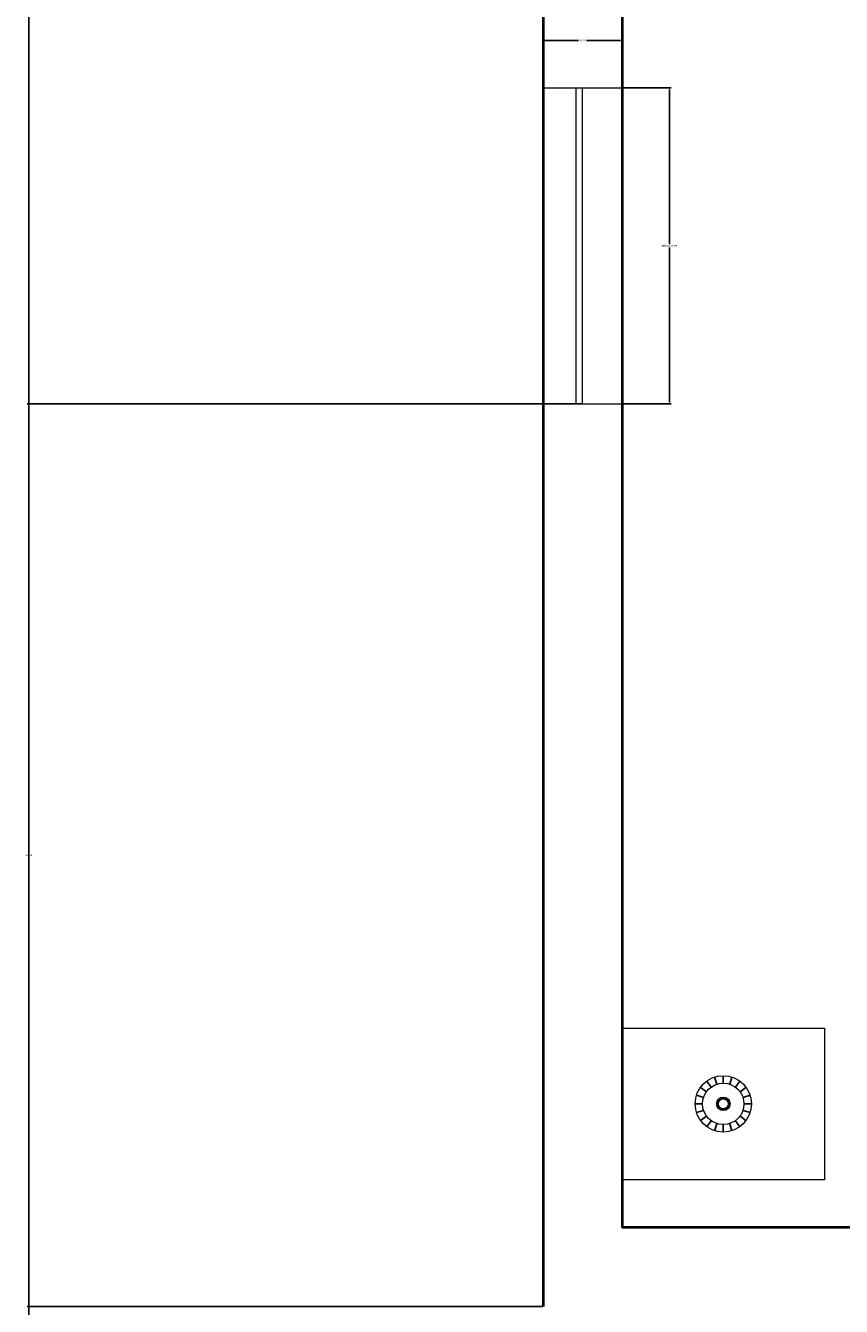
# Model space of a CAD drawing. Units: inches. Extents: x -46 to 1145, y -527 to 760.
# Tile 23 of 57: x -46 to 47, y 222 to 367. Entities that reach past the tile are written whole.
import ezdxf

# ---------------------------------------------------------------- set-up
doc = ezdxf.new("R2010")
doc.units = ezdxf.units.IN
doc.header["$MEASUREMENT"] = 0
for name, color, linetype, lineweight in [('A-ANNO-DIMS', 2, 'Continuous', 18), ('A-FURN', 2, 'Continuous', 13), ('WALLS', 4, 'Continuous', 40), ('WINDOWS', 240, 'Continuous', 20)]:
    doc.layers.add(name, color=color, linetype=linetype, lineweight=lineweight)
doc.layers.add('FURNTIURE', color=2, linetype='Continuous')
doc.styles.get("Standard").update_dxf_attribs({"font": 'arial.ttf'})
doc.dimstyles.get("Standard").update_dxf_attribs({"dimtxt": 0.18, "dimasz": 0.18, "dimexe": 0.18, "dimexo": 0.0625, "dimgap": 0.09, "dimtad": 0, "dimtih": 1, "dimtoh": 1, "dimdec": 0, "dimzin": 0, "dimdsep": 46, "dimlunit": 3, "dimtxsty": 'Standard', "dimcen": 0.09, "dimadec": 0, "dimazin": 0, "dimtfac": 1, "dimtdec": 0, "dimtofl": 0, "dimtmove": 0, "dimatfit": 3, "dimfxl": 1, "dimtolj": 1, "dimtzin": 0, "dimarcsym": 0})

# ---------------------------------------------------------------- blocks, each defined once
blk = doc.blocks.new('*U89')
at = {"layer": 'FURNTIURE'}
blk.add_line((0, 0.42), (0, -0.42), dxfattribs=at)
blk = doc.blocks.new('*U90')
at = {"layer": 'FURNTIURE', "transparency": 16777216}
for p, rotation in [((590.89, 507.4), 17.99999999999997), ((592.61, 507.4), 341.9999999999999), ((589.5, 506.39), 54), ((590.11, 507), 36), ((593.39, 507), 324), ((594.01, 506.39), 306), ((589.1, 505.61), 72), ((594.4, 505.61), 288), ((588.97, 504.75), 90), ((589.1, 503.89), 108), ((594.4, 503.89), 252), ((594.54, 504.75), 270), ((589.5, 503.11), 126), ((590.11, 502.49), 144), ((590.89, 502.1), 162), ((591.75, 501.96), 180), ((592.61, 502.1), 197.9999999999999), ((593.39, 502.49), 216), ((594.01, 503.11), 234)]:
    blk.add_blockref('*U89', p, dxfattribs=dict(at, rotation=rotation))
blk.add_blockref('*U89', (591.75, 507.53), dxfattribs=at)
blk = doc.blocks.new('*U87')
at = {"layer": 'FURNTIURE'}
blk.add_line((0, 0.1), (0, -0.1), dxfattribs=at)
blk = doc.blocks.new('*U88')
at = {"layer": 'FURNTIURE', "transparency": 16777216}
for p, rotation in [((141.27, 121.25), 72), ((141.36, 121.43), 54), ((141.51, 121.58), 35.99999999999999), ((141.7, 121.67), 17.99999999999998), ((142.11, 121.67), 342), ((142.3, 121.58), 324), ((142.44, 121.43), 306), ((142.54, 121.25), 288), ((141.23, 121.04), 90), ((141.27, 120.83), 108), ((141.36, 120.65), 126), ((141.51, 120.5), 144), ((141.7, 120.4), 162), ((141.9, 120.37), 180), ((142.11, 120.4), 198), ((142.3, 120.5), 216), ((142.44, 120.65), 234), ((142.54, 120.83), 252), ((142.57, 121.04), 270)]:
    blk.add_blockref('*U87', p, dxfattribs=dict(at, rotation=rotation))
blk.add_blockref('*U87', (141.9, 121.71), dxfattribs=at)
blk = doc.blocks.new('NIGHTSTAND')
blk.add_lwpolyline([(23.06, 0), (0, 0), (0, 17.28), (23.06, 17.28)], close=True)
for radius in [3.21, 2.36, 0.77, 0.567]:
    blk.add_circle((11.53, 8.64), radius)
for name, p in [('*U90', (-580.22, -496.1)), ('*U88', (-130.37, -112.4))]:
    blk.add_blockref(name, p)
blk = doc.blocks.new('WINDOW-36IN')
for p, q in [((0, 4.5), (0, 9)), ((0, 9), (0, 0)), ((36, 9), (36, 0)), ((0, 5.23), (36, 5.23)), ((0, 4.5), (36, 4.5))]:
    blk.add_line(p, q)
blk = doc.blocks.new('*D662')
at = {"layer": 'A-ANNO-DIMS', "color": 0, "lineweight": -2, "transparency": 16777216}
for p, q in [((21.63, 360.33), (27.14, 360.33)), ((26.96, 360.15), (26.96, 342.51)), ((26.96, 324.51), (26.96, 342.15)), ((21.63, 324.33), (27.14, 324.33))]:
    blk.add_line(p, q, dxfattribs=at)
at = {"layer": 'A-ANNO-DIMS', "color": 0, "transparency": 16777216}
for points in [[(26.93, 360.15), (26.99, 360.15), (26.96, 360.33)], [(26.93, 324.51), (26.99, 324.51), (26.96, 324.33)]]:
    blk.add_solid(points, dxfattribs=at)
at = {"layer": 'Defpoints', "color": 0, "transparency": 16777216}
for p in [(21.56, 360.33), (26.96, 360.33), (21.56, 324.33)]:
    blk.add_point(p, dxfattribs=at)
at = {"layer": 'A-ANNO-DIMS', "color": 0, "transparency": 16777216, "insert": (26.96, 342.33), "char_height": 0.18, "attachment_point": 5}
blk.add_mtext('\\A1;WINDOW 36 TYP.', dxfattribs=at)
blk = doc.blocks.new('*D663')
at = {"layer": 'A-ANNO-DIMS', "color": 0, "lineweight": -2, "transparency": 16777216}
for p, q in [((12.56, 360.39), (12.56, 365.91)), ((12.74, 365.73), (16.61, 365.73)), ((21.38, 365.73), (17.52, 365.73)), ((21.56, 360.39), (21.56, 365.91))]:
    blk.add_line(p, q, dxfattribs=at)
at = {"layer": 'A-ANNO-DIMS', "color": 0, "transparency": 16777216}
for points in [[(12.74, 365.76), (12.74, 365.7), (12.56, 365.73)], [(21.38, 365.76), (21.38, 365.7), (21.56, 365.73)]]:
    blk.add_solid(points, dxfattribs=at)
at = {"layer": 'Defpoints', "color": 0, "transparency": 16777216}
for p in [(12.56, 365.73), (12.56, 360.33), (21.56, 360.33)]:
    blk.add_point(p, dxfattribs=at)
at = {"layer": 'A-ANNO-DIMS', "color": 0, "transparency": 16777216, "insert": (17.06, 365.73), "char_height": 0.18, "attachment_point": 5}
blk.add_mtext('\\A1;9 TYP.', dxfattribs=at)
blk = doc.blocks.new('*D685')
at = {"layer": 'A-ANNO-DIMS', "color": 0, "lineweight": -2, "transparency": 16777216}
for p, q in [((183.5, 700.89), (-46.22, 700.89)), ((-46.04, 700.71), (-46.04, 116.39)), ((-46.04, -468.3), (-46.04, 116.02)), ((12.5, -468.48), (-46.22, -468.48))]:
    blk.add_line(p, q, dxfattribs=at)
at = {"layer": 'A-ANNO-DIMS', "color": 0, "transparency": 16777216}
for points in [[(-46.07, 700.71), (-46.01, 700.71), (-46.04, 700.89)], [(-46.07, -468.3), (-46.01, -468.3), (-46.04, -468.48)]]:
    blk.add_solid(points, dxfattribs=at)
at = {"layer": 'Defpoints', "color": 0, "transparency": 16777216}
for p in [(-46.04, 700.89), (183.56, 700.89), (12.56, -468.48)]:
    blk.add_point(p, dxfattribs=at)
at = {"layer": 'A-ANNO-DIMS', "color": 0, "transparency": 16777216, "insert": (-46.04, 116.2), "char_height": 0.18, "attachment_point": 5}
blk.add_mtext('\\A1;1169.4', dxfattribs=at)
blk = doc.blocks.new('*D698')
at = {"layer": 'A-ANNO-DIMS', "color": 0, "lineweight": -2, "transparency": 16777216}
for p, q in [((12.5, 324.33), (-46.22, 324.33)), ((-46.04, 324.15), (-46.04, 273.11)), ((-46.04, 221.7), (-46.04, 272.74)), ((12.5, 221.52), (-46.22, 221.52))]:
    blk.add_line(p, q, dxfattribs=at)
at = {"layer": 'A-ANNO-DIMS', "color": 0, "transparency": 16777216}
for points in [[(-46.07, 324.15), (-46.01, 324.15), (-46.04, 324.33)], [(-46.07, 221.7), (-46.01, 221.7), (-46.04, 221.52)]]:
    blk.add_solid(points, dxfattribs=at)
at = {"layer": 'Defpoints', "color": 0, "transparency": 16777216}
for p in [(-46.04, 324.33), (12.56, 324.33), (12.56, 221.52)]:
    blk.add_point(p, dxfattribs=at)
at = {"layer": 'A-ANNO-DIMS', "color": 0, "transparency": 16777216, "insert": (-46.04, 272.92), "char_height": 0.18, "attachment_point": 5}
blk.add_mtext('\\A1;102.81', dxfattribs=at)

msp = doc.modelspace()

# ---------------------------------------------------------------- linework, layer by layer
at = {"layer": 'WALLS'}
for p, q in [((12.5637, 659.5176), (12.5637, 221.5176)), ((21.5637, 379.5176), (21.5637, 230.5176)), ((183.5637, 230.5176), (21.5637, 230.5176))]:
    msp.add_line(p, q, dxfattribs=at)

# ---------------------------------------------------------------- block references
at = {"layer": 'A-FURN', "rotation": 180}
msp.add_blockref('NIGHTSTAND', (44.6243, 253.2307), dxfattribs=at)
at = {"layer": 'WINDOWS', "rotation": 90.00000000000006}
msp.add_blockref('WINDOW-36IN', (21.5633, 324.3306), dxfattribs=at)

# ---------------------------------------------------------------- dimensions: what is measured, and where the dimension line sits
at = {"layer": 'A-ANNO-DIMS'}
for base, p1, p2, override, picture, middle in [((-46.0363, 700.8886), (12.5637, -468.4824), (183.5637, 700.8886), {"dimdec": 1, "dimlfac": 1, "dimrnd": 0, "dimzin": 0, "dimdsep": 46, "dimlunit": 2}, '*D685', (-46.0363, 116.2031)), ((-46.0363, 324.3307), (12.5637, 221.5176), (12.5637, 324.3307), {"dimdec": 2, "dimlfac": 1, "dimrnd": 0, "dimzin": 0, "dimdsep": 46, "dimlunit": 2}, '*D698', (-46.0363, 272.9242))]:
    dim = msp.add_linear_dim(base=base, p1=p1, p2=p2, angle=90, dimstyle='Standard', override=override, dxfattribs=at)
    dim.commit()
    dim.dimension.update_dxf_attribs({"geometry": picture, "text_midpoint": middle})
for base, p1, p2, angle, text, picture, middle in [((12.5637, 365.7307), (21.5637, 360.3307), (12.5637, 360.3307), 180, '<> TYP.', '*D663', (17.0637, 365.7307)), ((26.9637, 360.3307), (21.5637, 324.3307), (21.5637, 360.3307), 90, 'WINDOW <> TYP.', '*D662', (26.9637, 342.3307))]:
    dim = msp.add_linear_dim(base=base, p1=p1, p2=p2, angle=angle, text=text, dimstyle='Standard', override={"dimdec": 0, "dimlfac": 1, "dimrnd": 0, "dimzin": 0, "dimdsep": 46, "dimlunit": 2}, dxfattribs=at)
    dim.commit()
    dim.dimension.update_dxf_attribs({"geometry": picture, "text_midpoint": middle})

doc.saveas('drawing.dxf')
